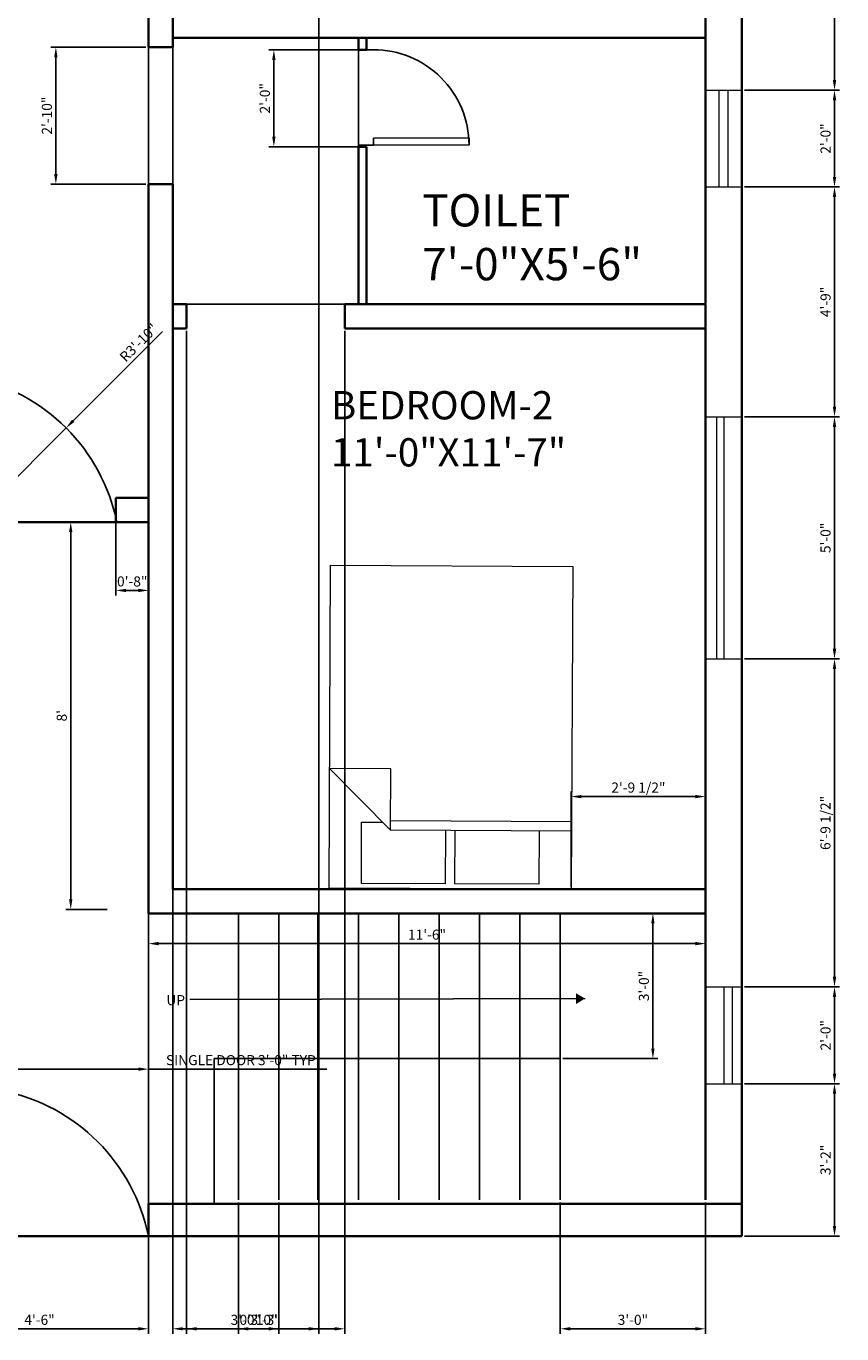
# Model space of a CAD drawing. Units: inches. Extents: x -2945 to -2182, y 3541 to 4172.
# Tile 4 of 5: x -2384 to -2182, y 3541 to 3865. Entities that reach past the tile are written whole.
import ezdxf

# ---------------------------------------------------------------- set-up
doc = ezdxf.new("R2010")
doc.units = ezdxf.units.IN
for name, color, linetype, lineweight in [('A-ANNO-DIMS', 2, 'Continuous', 18), ('A-ANNO-TEXT', 7, 'Continuous', 18), ('A-AREA-IDEN', 7, 'Continuous', 18), ('A-DOOR', 3, 'Continuous', 25), ('A-FLOR-STRS', 7, 'Continuous', 25), ('A-FURN', 9, 'Continuous', 18), ('A-GLAZ', 4, 'Continuous', 18), ('A-WALL', 7, 'Continuous', 35)]:
    doc.layers.add(name, color=color, linetype=linetype, lineweight=lineweight)
doc.styles.get("Standard").update_dxf_attribs({"font": 'arial.ttf'})
doc.dimstyles.new('ISO-25', dxfattribs={"dimtxt": 2.5, "dimasz": 2.5, "dimexe": 1.25, "dimexo": 0.625, "dimtad": 1, "dimdec": 0, "dimlunit": 3, "dimtxsty": 'Standard', "dimcen": 2.5, "dimadec": 0, "dimazin": 0, "dimtfac": 1, "dimtdec": 0, "dimtmove": 0, "dimatfit": 3, "dimfxl": 1, "dimarcsym": 0})

# ---------------------------------------------------------------- blocks, each defined once
blk = doc.blocks.new('Bed - Queen')
for p, q in [((0, -80.00003), (0, 0)), ((0, 0), (59.99999, 0)), ((59.99999, 0), (59.99999, -80.00003)), ((7.99999, -1.2), (28.79998, -1.2)), ((7.99999, -14.4), (7.99999, -1.2)), ((28.79998, -1.2), (28.79998, -14.4)), ((31.19999, -1.2), (51.99999, -1.2)), ((31.19999, -14.4), (31.19999, -1.2)), ((51.99999, -1.2), (51.99999, -16.4)), ((0, -14.4), (44.8, -14.4)), ((59.99999, -29.6), (44.8, -14.4)), ((44.8, -14.4), (44.8, -29.6)), ((44.8, -16.8), (0, -16.8)), ((51.99999, -16.4), (46.79936, -16.4)), ((44.8, -29.6), (59.99999, -29.6)), ((59.99999, -80.00003), (0, -80.00003))]:
    blk.add_line(p, q)
blk = doc.blocks.new('*U5')
for p, q in [((-600, 0), (-600, -100)), ((0, 0), (0, -100))]:
    blk.add_line(p, q)
blk.add_lwpolyline([(0, 0), (0, 600), (-43.75, 600), (-43.75, 0)], close=True)
blk.add_arc((0, 0), 600, 90, 180)
blk = doc.blocks.new('*D7')
at = {"layer": 'A-ANNO-DIMS', "color": 0, "lineweight": -2, "transparency": 16777216}
for p, q in [((-2354.05, 3636.42), (-2354.05, 3639.34)), ((-2218.55, 3638.09), (-2351.55, 3638.09)), ((-2216.05, 3636.42), (-2216.05, 3639.34))]:
    blk.add_line(p, q, dxfattribs=at)
at = {"layer": 'A-ANNO-DIMS', "color": 0, "transparency": 16777216}
for points in [[(-2351.55, 3638.51), (-2351.55, 3637.67), (-2354.05, 3638.09)], [(-2218.55, 3638.51), (-2218.55, 3637.67), (-2216.05, 3638.09)]]:
    blk.add_solid(points, dxfattribs=at)
at = {"layer": 'Defpoints', "color": 0, "transparency": 16777216}
for p in [(-2354.05, 3638.09), (-2354.05, 3635.8), (-2216.05, 3635.8)]:
    blk.add_point(p, dxfattribs=at)
at = {"layer": 'A-ANNO-DIMS', "color": 0, "transparency": 16777216, "insert": (-2285.05, 3639.99), "char_height": 2.5, "attachment_point": 5}
blk.add_mtext('11\'-6"', dxfattribs=at)
blk = doc.blocks.new('*D8')
at = {"layer": 'A-ANNO-DIMS', "color": 0, "lineweight": -2, "transparency": 16777216}
for p, q in [((-2362.73, 3742.58), (-2374.56, 3742.58)), ((-2373.31, 3740.08), (-2373.31, 3649.07)), ((-2364.29, 3646.57), (-2374.56, 3646.57))]:
    blk.add_line(p, q, dxfattribs=at)
at = {"layer": 'A-ANNO-DIMS', "color": 0, "transparency": 16777216}
for points in [[(-2373.73, 3740.08), (-2372.9, 3740.08), (-2373.31, 3742.58)], [(-2373.73, 3649.07), (-2372.9, 3649.07), (-2373.31, 3646.57)]]:
    blk.add_solid(points, dxfattribs=at)
at = {"layer": 'Defpoints', "color": 0, "transparency": 16777216}
for p in [(-2362.11, 3742.58), (-2373.31, 3646.57), (-2363.67, 3646.57)]:
    blk.add_point(p, dxfattribs=at)
at = {"layer": 'A-ANNO-DIMS', "color": 0, "transparency": 16777216, "insert": (-2375.22, 3694.57), "char_height": 2.5, "attachment_point": 5, "rotation": 90}
blk.add_mtext("8'", dxfattribs=at)
blk = doc.blocks.new('DOOR-SINGLE-36IN')
for p, q in [((0, 0), (0, 36)), ((1, 0), (1, 36))]:
    blk.add_line(p, q)
blk.add_arc((-9.18, -9.18), 46.1, 11.4852, 78.5148)
blk = doc.blocks.new('*D18')
at = {"layer": 'A-ANNO-DIMS', "color": 0, "lineweight": -2, "transparency": 16777216}
for p, q in [((-2390.05, 3602.2), (-2390.05, 3608.23)), ((-2354.05, 3602.2), (-2354.05, 3608.23)), ((-2387.55, 3606.98), (-2356.55, 3606.98)), ((-2354.05, 3606.98), (-2309.84, 3606.98))]:
    blk.add_line(p, q, dxfattribs=at)
at = {"layer": 'A-ANNO-DIMS', "color": 0, "transparency": 16777216}
for points in [[(-2387.55, 3607.39), (-2387.55, 3606.56), (-2390.05, 3606.98)], [(-2356.55, 3607.39), (-2356.55, 3606.56), (-2354.05, 3606.98)]]:
    blk.add_solid(points, dxfattribs=at)
at = {"layer": 'Defpoints', "color": 0, "transparency": 16777216}
for p in [(-2354.05, 3606.98), (-2390.05, 3601.58), (-2354.05, 3601.58)]:
    blk.add_point(p, dxfattribs=at)
at = {"layer": 'A-ANNO-DIMS', "color": 0, "transparency": 16777216, "insert": (-2330.7, 3608.89), "char_height": 2.5, "attachment_point": 5}
blk.add_mtext('SINGLE DOOR 3\'-0" TYP.', dxfattribs=at)
blk = doc.blocks.new('*D33')
at = {"layer": 'A-ANNO-DIMS', "color": 0, "lineweight": -2, "transparency": 16777216}
for p, q in [((-2206.42, 3603.38), (-2182.85, 3603.38)), ((-2184.1, 3568.08), (-2184.1, 3600.88)), ((-2206.42, 3565.58), (-2182.85, 3565.58))]:
    blk.add_line(p, q, dxfattribs=at)
at = {"layer": 'A-ANNO-DIMS', "color": 0, "transparency": 16777216}
for points in [[(-2184.52, 3600.88), (-2183.68, 3600.88), (-2184.1, 3603.38)], [(-2184.52, 3568.08), (-2183.68, 3568.08), (-2184.1, 3565.58)]]:
    blk.add_solid(points, dxfattribs=at)
at = {"layer": 'Defpoints', "color": 0, "transparency": 16777216}
for p in [(-2207.05, 3603.38), (-2184.1, 3603.38), (-2207.05, 3565.58)]:
    blk.add_point(p, dxfattribs=at)
at = {"layer": 'A-ANNO-DIMS', "color": 0, "transparency": 16777216, "insert": (-2186, 3584.48), "char_height": 2.5, "attachment_point": 5, "rotation": 90}
blk.add_mtext('3\'-2"', dxfattribs=at)
blk = doc.blocks.new('*D34')
at = {"layer": 'A-ANNO-DIMS', "color": 0, "lineweight": -2, "transparency": 16777216}
for p, q in [((-2206.42, 3627.38), (-2182.85, 3627.38)), ((-2184.1, 3605.88), (-2184.1, 3624.88)), ((-2206.42, 3603.38), (-2182.85, 3603.38))]:
    blk.add_line(p, q, dxfattribs=at)
at = {"layer": 'A-ANNO-DIMS', "color": 0, "transparency": 16777216}
for points in [[(-2184.52, 3624.88), (-2183.68, 3624.88), (-2184.1, 3627.38)], [(-2184.52, 3605.88), (-2183.68, 3605.88), (-2184.1, 3603.38)]]:
    blk.add_solid(points, dxfattribs=at)
at = {"layer": 'Defpoints', "color": 0, "transparency": 16777216}
for p in [(-2207.05, 3627.38), (-2184.1, 3627.38), (-2207.05, 3603.38)]:
    blk.add_point(p, dxfattribs=at)
at = {"layer": 'A-ANNO-DIMS', "color": 0, "transparency": 16777216, "insert": (-2186, 3615.38), "char_height": 2.5, "attachment_point": 5, "rotation": 90}
blk.add_mtext('2\'-0"', dxfattribs=at)
blk = doc.blocks.new('*D35')
at = {"layer": 'A-ANNO-DIMS', "color": 0, "lineweight": -2, "transparency": 16777216}
for p, q in [((-2206.42, 3708.65), (-2182.85, 3708.65)), ((-2184.1, 3629.88), (-2184.1, 3706.15)), ((-2206.42, 3627.38), (-2182.85, 3627.38))]:
    blk.add_line(p, q, dxfattribs=at)
at = {"layer": 'A-ANNO-DIMS', "color": 0, "transparency": 16777216}
for points in [[(-2184.52, 3706.15), (-2183.68, 3706.15), (-2184.1, 3708.65)], [(-2184.52, 3629.88), (-2183.68, 3629.88), (-2184.1, 3627.38)]]:
    blk.add_solid(points, dxfattribs=at)
at = {"layer": 'Defpoints', "color": 0, "transparency": 16777216}
for p in [(-2207.05, 3708.65), (-2184.1, 3708.65), (-2207.05, 3627.38)]:
    blk.add_point(p, dxfattribs=at)
at = {"layer": 'A-ANNO-DIMS', "color": 0, "transparency": 16777216, "insert": (-2186.02, 3668.01), "char_height": 2.5, "attachment_point": 5, "rotation": 90}
blk.add_mtext('6\'-9 1/2"', dxfattribs=at)
blk = doc.blocks.new('*D36')
at = {"layer": 'A-ANNO-DIMS', "color": 0, "lineweight": -2, "transparency": 16777216}
for p, q in [((-2206.42, 3768.65), (-2182.85, 3768.65)), ((-2184.1, 3711.15), (-2184.1, 3766.15)), ((-2206.42, 3708.65), (-2182.85, 3708.65))]:
    blk.add_line(p, q, dxfattribs=at)
at = {"layer": 'A-ANNO-DIMS', "color": 0, "transparency": 16777216}
for points in [[(-2184.52, 3766.15), (-2183.68, 3766.15), (-2184.1, 3768.65)], [(-2184.52, 3711.15), (-2183.68, 3711.15), (-2184.1, 3708.65)]]:
    blk.add_solid(points, dxfattribs=at)
at = {"layer": 'Defpoints', "color": 0, "transparency": 16777216}
for p in [(-2207.05, 3768.65), (-2184.1, 3768.65), (-2207.05, 3708.65)]:
    blk.add_point(p, dxfattribs=at)
at = {"layer": 'A-ANNO-DIMS', "color": 0, "transparency": 16777216, "insert": (-2186, 3738.65), "char_height": 2.5, "attachment_point": 5, "rotation": 90}
blk.add_mtext('5\'-0"', dxfattribs=at)
blk = doc.blocks.new('*D37')
at = {"layer": 'A-ANNO-DIMS', "color": 0, "lineweight": -2, "transparency": 16777216}
for p, q in [((-2206.42, 3825.62), (-2182.85, 3825.62)), ((-2184.1, 3771.15), (-2184.1, 3823.12)), ((-2206.42, 3768.65), (-2182.85, 3768.65))]:
    blk.add_line(p, q, dxfattribs=at)
at = {"layer": 'A-ANNO-DIMS', "color": 0, "transparency": 16777216}
for points in [[(-2184.52, 3823.12), (-2183.68, 3823.12), (-2184.1, 3825.62)], [(-2184.52, 3771.15), (-2183.68, 3771.15), (-2184.1, 3768.65)]]:
    blk.add_solid(points, dxfattribs=at)
at = {"layer": 'Defpoints', "color": 0, "transparency": 16777216}
for p in [(-2207.05, 3825.62), (-2184.1, 3825.62), (-2207.05, 3768.65)]:
    blk.add_point(p, dxfattribs=at)
at = {"layer": 'A-ANNO-DIMS', "color": 0, "transparency": 16777216, "insert": (-2186, 3797.13), "char_height": 2.5, "attachment_point": 5, "rotation": 90}
blk.add_mtext('4\'-9"', dxfattribs=at)
blk = doc.blocks.new('*D38')
at = {"layer": 'A-ANNO-DIMS', "color": 0, "lineweight": -2, "transparency": 16777216}
for p, q in [((-2206.42, 3849.62), (-2182.85, 3849.62)), ((-2184.1, 3828.12), (-2184.1, 3847.12)), ((-2206.42, 3825.62), (-2182.85, 3825.62))]:
    blk.add_line(p, q, dxfattribs=at)
at = {"layer": 'A-ANNO-DIMS', "color": 0, "transparency": 16777216}
for points in [[(-2184.52, 3847.12), (-2183.68, 3847.12), (-2184.1, 3849.62)], [(-2184.52, 3828.12), (-2183.68, 3828.12), (-2184.1, 3825.62)]]:
    blk.add_solid(points, dxfattribs=at)
at = {"layer": 'Defpoints', "color": 0, "transparency": 16777216}
for p in [(-2207.05, 3849.62), (-2184.1, 3849.62), (-2207.05, 3825.62)]:
    blk.add_point(p, dxfattribs=at)
at = {"layer": 'A-ANNO-DIMS', "color": 0, "transparency": 16777216, "insert": (-2186, 3837.62), "char_height": 2.5, "attachment_point": 5, "rotation": 90}
blk.add_mtext('2\'-0"', dxfattribs=at)
blk = doc.blocks.new('*D39')
at = {"layer": 'A-ANNO-DIMS', "color": 0, "lineweight": -2, "transparency": 16777216}
for p, q in [((-2206.42, 3918.54), (-2182.85, 3918.54)), ((-2184.1, 3852.12), (-2184.1, 3916.04)), ((-2206.42, 3849.62), (-2182.85, 3849.62))]:
    blk.add_line(p, q, dxfattribs=at)
at = {"layer": 'A-ANNO-DIMS', "color": 0, "transparency": 16777216}
for points in [[(-2184.52, 3916.04), (-2183.68, 3916.04), (-2184.1, 3918.54)], [(-2184.52, 3852.12), (-2183.68, 3852.12), (-2184.1, 3849.62)]]:
    blk.add_solid(points, dxfattribs=at)
at = {"layer": 'Defpoints', "color": 0, "transparency": 16777216}
for p in [(-2207.05, 3918.54), (-2184.1, 3918.54), (-2207.05, 3849.62)]:
    blk.add_point(p, dxfattribs=at)
at = {"layer": 'A-ANNO-DIMS', "color": 0, "transparency": 16777216, "insert": (-2186, 3884.08), "char_height": 2.5, "attachment_point": 5, "rotation": 90}
blk.add_mtext('5\'-9"', dxfattribs=at)
blk = doc.blocks.new('*D41')
at = {"layer": 'A-ANNO-DIMS', "color": 0, "lineweight": -2, "transparency": 16777216}
for p, q in [((-2408.05, 3920.95), (-2408.05, 3541.38)), ((-2354.05, 3920.95), (-2354.05, 3541.38)), ((-2405.55, 3542.63), (-2356.55, 3542.63))]:
    blk.add_line(p, q, dxfattribs=at)
at = {"layer": 'A-ANNO-DIMS', "color": 0, "transparency": 16777216}
for points in [[(-2405.55, 3543.04), (-2405.55, 3542.21), (-2408.05, 3542.63)], [(-2356.55, 3543.04), (-2356.55, 3542.21), (-2354.05, 3542.63)]]:
    blk.add_solid(points, dxfattribs=at)
at = {"layer": 'Defpoints', "color": 0, "transparency": 16777216}
for p in [(-2408.05, 3921.58), (-2354.05, 3921.58), (-2354.05, 3542.63)]:
    blk.add_point(p, dxfattribs=at)
at = {"layer": 'A-ANNO-DIMS', "color": 0, "transparency": 16777216, "insert": (-2381.05, 3544.53), "char_height": 2.5, "attachment_point": 5}
blk.add_mtext('4\'-6"', dxfattribs=at)
blk = doc.blocks.new('*D48')
at = {"layer": 'A-ANNO-DIMS', "color": 0, "lineweight": -2, "transparency": 16777216}
for p, q in [((-2300.67, 3859.61), (-2324.24, 3859.61)), ((-2323, 3838.08), (-2323, 3857.11)), ((-2300.67, 3835.57), (-2324.25, 3835.58))]:
    blk.add_line(p, q, dxfattribs=at)
at = {"layer": 'A-ANNO-DIMS', "color": 0, "transparency": 16777216}
for points in [[(-2323.41, 3857.11), (-2322.58, 3857.11), (-2322.99, 3859.61)], [(-2323.41, 3838.08), (-2322.58, 3838.08), (-2323, 3835.58)]]:
    blk.add_solid(points, dxfattribs=at)
at = {"layer": 'Defpoints', "color": 0, "transparency": 16777216}
for p in [(-2322.99, 3859.61), (-2300.04, 3859.61), (-2300.05, 3835.57)]:
    blk.add_point(p, dxfattribs=at)
at = {"layer": 'A-ANNO-DIMS', "color": 0, "transparency": 16777216, "insert": (-2324.9, 3847.6), "char_height": 2.5, "attachment_point": 5, "rotation": 89.9911}
blk.add_mtext('2\'-0"', dxfattribs=at)
blk = doc.blocks.new('*D50')
at = {"layer": 'A-ANNO-DIMS', "color": 0, "lineweight": -2, "transparency": 16777216}
for p, q in [((-2354.67, 3860.25), (-2378.25, 3860.25)), ((-2377, 3828.85), (-2377, 3857.75)), ((-2354.67, 3826.35), (-2378.25, 3826.35))]:
    blk.add_line(p, q, dxfattribs=at)
at = {"layer": 'A-ANNO-DIMS', "color": 0, "transparency": 16777216}
for points in [[(-2377.42, 3857.75), (-2376.58, 3857.75), (-2377, 3860.25)], [(-2377.42, 3828.85), (-2376.58, 3828.85), (-2377, 3826.35)]]:
    blk.add_solid(points, dxfattribs=at)
at = {"layer": 'Defpoints', "color": 0, "transparency": 16777216}
for p in [(-2377, 3860.25), (-2354.05, 3860.25), (-2354.05, 3826.35)]:
    blk.add_point(p, dxfattribs=at)
at = {"layer": 'A-ANNO-DIMS', "color": 0, "transparency": 16777216, "insert": (-2378.9, 3843.3), "char_height": 2.5, "attachment_point": 5, "rotation": 90}
blk.add_mtext('2\'-10"', dxfattribs=at)
blk = doc.blocks.new('*D51')
at = {"layer": 'A-ANNO-DIMS', "color": 0, "lineweight": -2, "transparency": 16777216}
for p, q in [((-2344.65, 3789.95), (-2344.65, 3541.38)), ((-2305.42, 3789.95), (-2305.42, 3541.38)), ((-2342.15, 3542.63), (-2307.92, 3542.63))]:
    blk.add_line(p, q, dxfattribs=at)
at = {"layer": 'A-ANNO-DIMS', "color": 0, "transparency": 16777216}
for points in [[(-2342.15, 3543.04), (-2342.15, 3542.21), (-2344.65, 3542.63)], [(-2307.92, 3543.04), (-2307.92, 3542.21), (-2305.42, 3542.63)]]:
    blk.add_solid(points, dxfattribs=at)
at = {"layer": 'Defpoints', "color": 0, "transparency": 16777216}
for p in [(-2344.65, 3790.58), (-2305.42, 3790.58), (-2305.42, 3542.63)]:
    blk.add_point(p, dxfattribs=at)
at = {"layer": 'A-ANNO-DIMS', "color": 0, "transparency": 16777216, "insert": (-2325.04, 3544.53), "char_height": 2.5, "attachment_point": 5}
blk.add_mtext('3\'-3"', dxfattribs=at)
blk = doc.blocks.new('*D52')
at = {"layer": 'A-ANNO-DIMS', "color": 0, "lineweight": -2, "transparency": 16777216}
for p, q in [((-2252.05, 3573.95), (-2252.05, 3541.38)), ((-2216.05, 3573.95), (-2216.05, 3541.38)), ((-2249.55, 3542.63), (-2218.55, 3542.63))]:
    blk.add_line(p, q, dxfattribs=at)
at = {"layer": 'A-ANNO-DIMS', "color": 0, "transparency": 16777216}
for points in [[(-2249.55, 3543.04), (-2249.55, 3542.21), (-2252.05, 3542.63)], [(-2218.55, 3543.04), (-2218.55, 3542.21), (-2216.05, 3542.63)]]:
    blk.add_solid(points, dxfattribs=at)
at = {"layer": 'Defpoints', "color": 0, "transparency": 16777216}
for p in [(-2252.05, 3574.58), (-2216.05, 3574.58), (-2216.05, 3542.63)]:
    blk.add_point(p, dxfattribs=at)
at = {"layer": 'A-ANNO-DIMS', "color": 0, "transparency": 16777216, "insert": (-2234.05, 3544.53), "char_height": 2.5, "attachment_point": 5}
blk.add_mtext('3\'-0"', dxfattribs=at)
blk = doc.blocks.new('*D53')
at = {"layer": 'A-ANNO-DIMS', "color": 0, "lineweight": -2, "transparency": 16777216}
for p, q in [((-2331.79, 3573.95), (-2331.79, 3541.38)), ((-2321.79, 3573.95), (-2321.79, 3541.38)), ((-2329.29, 3542.63), (-2324.29, 3542.63))]:
    blk.add_line(p, q, dxfattribs=at)
at = {"layer": 'A-ANNO-DIMS', "color": 0, "transparency": 16777216}
for points in [[(-2329.29, 3543.04), (-2329.29, 3542.21), (-2331.79, 3542.63)], [(-2324.29, 3543.04), (-2324.29, 3542.21), (-2321.79, 3542.63)]]:
    blk.add_solid(points, dxfattribs=at)
at = {"layer": 'Defpoints', "color": 0, "transparency": 16777216}
for p in [(-2331.79, 3574.58), (-2321.79, 3574.58), (-2321.79, 3542.63)]:
    blk.add_point(p, dxfattribs=at)
at = {"layer": 'A-ANNO-DIMS', "color": 0, "transparency": 16777216, "insert": (-2326.79, 3544.53), "char_height": 2.5, "attachment_point": 5}
blk.add_mtext('0\'-10"', dxfattribs=at)
blk = doc.blocks.new('*D54')
at = {"layer": 'A-ANNO-DIMS', "color": 0, "lineweight": -2, "transparency": 16777216}
for p, q in [((-2251.42, 3645.58), (-2227.85, 3645.58)), ((-2229.1, 3643.08), (-2229.1, 3612.08)), ((-2251.42, 3609.58), (-2227.85, 3609.58))]:
    blk.add_line(p, q, dxfattribs=at)
at = {"layer": 'A-ANNO-DIMS', "color": 0, "transparency": 16777216}
for points in [[(-2229.52, 3643.08), (-2228.68, 3643.08), (-2229.1, 3645.58)], [(-2229.52, 3612.08), (-2228.68, 3612.08), (-2229.1, 3609.58)]]:
    blk.add_solid(points, dxfattribs=at)
at = {"layer": 'Defpoints', "color": 0, "transparency": 16777216}
for p in [(-2252.05, 3645.58), (-2252.05, 3609.58), (-2229.1, 3609.58)]:
    blk.add_point(p, dxfattribs=at)
at = {"layer": 'A-ANNO-DIMS', "color": 0, "transparency": 16777216, "insert": (-2231, 3627.58), "char_height": 2.5, "attachment_point": 5, "rotation": 90}
blk.add_mtext('3\'-0"', dxfattribs=at)
blk = doc.blocks.new('*D55')
at = {"layer": 'A-ANNO-DIMS', "color": 0, "lineweight": -2, "transparency": 16777216}
for p, q in [((-2348.05, 3999.95), (-2348.05, 3541.38)), ((-2311.84, 3998.65), (-2311.84, 3541.38)), ((-2345.55, 3542.63), (-2314.34, 3542.63))]:
    blk.add_line(p, q, dxfattribs=at)
at = {"layer": 'A-ANNO-DIMS', "color": 0, "transparency": 16777216}
for points in [[(-2345.55, 3543.04), (-2345.55, 3542.21), (-2348.05, 3542.63)], [(-2314.34, 3543.04), (-2314.34, 3542.21), (-2311.84, 3542.63)]]:
    blk.add_solid(points, dxfattribs=at)
at = {"layer": 'Defpoints', "color": 0, "transparency": 16777216}
for p in [(-2348.05, 4000.58), (-2311.84, 3999.28), (-2311.84, 3542.63)]:
    blk.add_point(p, dxfattribs=at)
at = {"layer": 'A-ANNO-DIMS', "color": 0, "transparency": 16777216, "insert": (-2329.94, 3544.53), "char_height": 2.5, "attachment_point": 5}
blk.add_mtext('3\'-0"', dxfattribs=at)
blk = doc.blocks.new('*D56')
at = {"layer": 'A-ANNO-DIMS', "color": 0, "lineweight": -2, "transparency": 16777216}
for p, q in [((-2249.33, 3652.2), (-2249.33, 3675.78)), ((-2216.05, 3652.2), (-2216.05, 3675.78)), ((-2246.83, 3674.53), (-2218.55, 3674.53))]:
    blk.add_line(p, q, dxfattribs=at)
at = {"layer": 'A-ANNO-DIMS', "color": 0, "transparency": 16777216}
for points in [[(-2246.83, 3674.94), (-2246.83, 3674.11), (-2249.33, 3674.53)], [(-2218.55, 3674.94), (-2218.55, 3674.11), (-2216.05, 3674.53)]]:
    blk.add_solid(points, dxfattribs=at)
at = {"layer": 'Defpoints', "color": 0, "transparency": 16777216}
for p in [(-2216.05, 3674.53), (-2249.33, 3651.58), (-2216.05, 3651.58)]:
    blk.add_point(p, dxfattribs=at)
at = {"layer": 'A-ANNO-DIMS', "color": 0, "transparency": 16777216, "insert": (-2232.69, 3676.44), "char_height": 2.5, "attachment_point": 5}
blk.add_mtext('2\'-9 1/2"', dxfattribs=at)
blk = doc.blocks.new('*D57')
at = {"layer": 'A-ANNO-DIMS', "color": 0, "lineweight": -2, "transparency": 16777216}
for p, q in [((-2362.11, 3747.95), (-2362.11, 3724.38)), ((-2354.05, 3747.95), (-2354.05, 3724.38)), ((-2356.55, 3725.63), (-2359.61, 3725.63))]:
    blk.add_line(p, q, dxfattribs=at)
at = {"layer": 'A-ANNO-DIMS', "color": 0, "transparency": 16777216}
for points in [[(-2359.61, 3726.04), (-2359.61, 3725.21), (-2362.11, 3725.63)], [(-2356.55, 3726.04), (-2356.55, 3725.21), (-2354.05, 3725.63)]]:
    blk.add_solid(points, dxfattribs=at)
at = {"layer": 'Defpoints', "color": 0, "transparency": 16777216}
for p in [(-2362.11, 3748.58), (-2354.05, 3748.58), (-2362.11, 3725.63)]:
    blk.add_point(p, dxfattribs=at)
at = {"layer": 'A-ANNO-DIMS', "color": 0, "transparency": 16777216, "insert": (-2358.08, 3727.53), "char_height": 2.5, "attachment_point": 5}
blk.add_mtext('0\'-8"', dxfattribs=at)
blk = doc.blocks.new('*D77')
at = {"layer": 'A-ANNO-DIMS', "color": 0, "lineweight": -2, "transparency": 16777216}
for p, q in [((-2350.58, 3789.78), (-2372.69, 3767.66)), ((-2407.06, 3733.29), (-2374.46, 3765.89))]:
    blk.add_line(p, q, dxfattribs=at)
at = {"layer": 'A-ANNO-DIMS', "color": 0, "transparency": 16777216}
blk.add_solid([(-2372.99, 3767.96), (-2372.4, 3767.37), (-2374.46, 3765.89)], dxfattribs=at)
at = {"layer": 'Defpoints', "color": 0, "transparency": 16777216}
for p in [(-2374.46, 3765.89), (-2407.06, 3733.29)]:
    blk.add_point(p, dxfattribs=at)
at = {"layer": 'A-ANNO-DIMS', "color": 0, "transparency": 16777216, "insert": (-2356.24, 3786.8), "char_height": 2.5, "attachment_point": 5, "rotation": 44.9998}
blk.add_mtext('R3\'-10"', dxfattribs=at)

msp = doc.modelspace()

# ---------------------------------------------------------------- linework, layer by layer
at = {"layer": 'A-DOOR'}
for p, q in [((-2302.02, 3835.57), (-2302.02, 3859.57)), ((-2344.65, 3796.58), (-2305.42, 3796.58))]:
    msp.add_line(p, q, dxfattribs=at)
at = {"layer": 'A-FLOR-STRS'}
for p, q in [((-2331.79, 3645.58), (-2331.79, 3574.58)), ((-2321.79, 3645.58), (-2321.79, 3574.58)), ((-2312.11, 3645.58), (-2312.11, 3574.58)), ((-2302.02, 3645.58), (-2302.02, 3574.58)), ((-2292.05, 3645.58), (-2292.05, 3574.58)), ((-2282.05, 3645.58), (-2282.05, 3574.58)), ((-2272.05, 3645.58), (-2272.05, 3574.58)), ((-2272.05, 3645.58), (-2272.05, 3574.58)), ((-2262.05, 3645.58), (-2262.05, 3574.58)), ((-2262.05, 3645.58), (-2262.05, 3574.58)), ((-2252.05, 3645.58), (-2252.05, 3574.58)), ((-2343.79, 3624.21), (-2245.91, 3624.47)), ((-2331.79, 3609.58), (-2337.77, 3609.58)), ((-2337.77, 3609.58), (-2337.77, 3573.58)), ((-2252.05, 3609.58), (-2331.79, 3609.58))]:
    msp.add_line(p, q, dxfattribs=at)
msp.add_lwpolyline([(-2245.91, 3624.47, 0, 2.68, 0), (-2248.15, 3624.46, 2.68, 2.68, 0)], format="xyseb", dxfattribs=at)
at = {"layer": 'A-GLAZ'}
for p, q in [((-2216.05, 3849.62), (-2207.05, 3849.62)), ((-2212.73, 3849.62), (-2212.73, 3825.62)), ((-2210.56, 3849.62), (-2210.56, 3825.62)), ((-2216.05, 3825.62), (-2207.05, 3825.62)), ((-2216.05, 3768.65), (-2207.05, 3768.65)), ((-2213.37, 3768.65), (-2213.37, 3708.65)), ((-2211.55, 3768.65), (-2211.55, 3708.65)), ((-2216.05, 3708.65), (-2207.05, 3708.65)), ((-2216.05, 3627.38), (-2207.05, 3627.38)), ((-2211.55, 3627.38), (-2211.55, 3603.38)), ((-2209.48, 3627.38), (-2209.48, 3603.38)), ((-2216.05, 3603.38), (-2207.05, 3603.38))]:
    msp.add_line(p, q, dxfattribs=at)
at = {"layer": 'A-WALL'}
for p, q in [((-2207.05, 4009.58), (-2207.05, 3565.58)), ((-2216.05, 4000.58), (-2216.05, 3574.58)), ((-2354.05, 3860.25), (-2354.05, 3872.23)), ((-2348.05, 3860.25), (-2348.05, 3872.23)), ((-2354.05, 3860.25), (-2348.05, 3860.25)), ((-2348.05, 3862.58), (-2216.05, 3862.58)), ((-2302.02, 3862.58), (-2302.02, 3859.57)), ((-2300.05, 3862.58), (-2300.05, 3859.57)), ((-2302.02, 3859.57), (-2300.05, 3859.57)), ((-2302.02, 3835.57), (-2300.05, 3835.57)), ((-2302.02, 3835.57), (-2302.02, 3796.58)), ((-2300.05, 3835.57), (-2300.05, 3796.58)), ((-2354.05, 3645.58), (-2354.05, 3826.35)), ((-2354.05, 3826.35), (-2348.05, 3826.35)), ((-2348.05, 3651.58), (-2348.05, 3826.35)), ((-2348.05, 3796.58), (-2344.65, 3796.58)), ((-2344.65, 3796.58), (-2344.65, 3790.58)), ((-2305.42, 3796.58), (-2305.42, 3790.58)), ((-2305.42, 3796.58), (-2216.05, 3796.58)), ((-2348.05, 3790.58), (-2344.65, 3790.58)), ((-2305.42, 3790.58), (-2216.05, 3790.58)), ((-2362.11, 3748.58), (-2362.11, 3742.58)), ((-2362.11, 3748.58), (-2354.05, 3748.58)), ((-2522.05, 3742.58), (-2354.05, 3742.58)), ((-2348.05, 3651.58), (-2216.05, 3651.58)), ((-2354.05, 3645.58), (-2216.05, 3645.58)), ((-2207.05, 3573.58), (-2354.05, 3573.58)), ((-2354.05, 3573.58), (-2354.05, 3565.58)), ((-2207.05, 3565.58), (-2531.05, 3565.58))]:
    msp.add_line(p, q, dxfattribs=at)

# ---------------------------------------------------------------- block references
at = {"layer": 'A-DOOR', "xscale": 0.0393700787401575, "yscale": 0.0393700787401575, "zscale": 0.0393700787401575, "rotation": 270.1211645851394}
msp.add_blockref('*U5', (-2298.27, 3835.99), dxfattribs=at)
at = {"layer": 'A-DOOR'}
for p in [(-2397.88, 3742.47), (-2390.05, 3565.57)]:
    msp.add_blockref('DOOR-SINGLE-36IN', p, dxfattribs=at)
at = {"layer": 'A-FURN', "rotation": 179.7397650528711}
msp.add_blockref('Bed - Queen', (-2249.33, 3651.58), dxfattribs=at)

# ---------------------------------------------------------------- texts
at = {"layer": 'A-ANNO-TEXT', "insert": (-2349.62, 3625.33), "char_height": 2.5, "attachment_point": 1}
msp.add_mtext_dynamic_manual_height_columns('UP', width=10.3268, gutter_width=12.5, heights=[0], dxfattribs=at)
at = {"layer": 'A-AREA-IDEN', "attachment_point": 1}
for s, width, heights, insert, char_height in [('TOILET\\P7\'-0"X5\'-6"', 51.4369, [29.22], (-2286.25, 3823.83), 8), ('BEDROOM-2\\P11\'-0"X11\'-7"', 36.5253, [0], (-2308.85, 3775.02), 7)]:
    msp.add_mtext_dynamic_manual_height_columns(s, width=width, gutter_width=12.5, heights=heights, dxfattribs=dict(at, insert=insert, char_height=char_height))

# ---------------------------------------------------------------- dimensions: what is measured, and where the dimension line sits
at = {"layer": 'A-ANNO-DIMS'}
for base, p1, p2, override, picture, middle in [((-2311.84, 3542.63), (-2348.05, 4000.58), (-2311.84, 3999.28), {"dimdec": 1, "dimlfac": 1, "dimrnd": 0, "dimzin": 1, "dimdsep": 46, "dimlunit": 4, "dimfrac": 2}, '*D55', (-2329.94, 3544.53)), ((-2354.05, 3542.63), (-2408.05, 3921.58), (-2354.05, 3921.58), {"dimdec": 1, "dimlfac": 1, "dimrnd": 0, "dimzin": 1, "dimdsep": 46, "dimlunit": 4, "dimfrac": 2}, '*D41', (-2381.05, 3544.53)), ((-2305.42, 3542.63), (-2344.65, 3790.58), (-2305.42, 3790.58), {"dimdec": 1, "dimlfac": 1, "dimrnd": 0, "dimzin": 1, "dimdsep": 46, "dimlunit": 4, "dimfrac": 2}, '*D51', (-2325.04, 3544.53)), ((-2216.05, 3674.53), (-2249.33, 3651.58), (-2216.05, 3651.58), {"dimdec": 1, "dimlfac": 1, "dimrnd": 0, "dimzin": 1, "dimdsep": 46, "dimlunit": 4, "dimfrac": 2}, '*D56', (-2232.69, 3676.44)), ((-2354.05, 3638.09), (-2216.05, 3635.8), (-2354.05, 3635.8), {"dimclrd": 0, "dimclre": 0, "dimclrt": 0}, '*D7', (-2285.05, 3639.99)), ((-2321.79, 3542.63), (-2331.79, 3574.58), (-2321.79, 3574.58), {"dimdec": 1, "dimlfac": 1, "dimrnd": 0, "dimzin": 1, "dimdsep": 46, "dimlunit": 4, "dimfrac": 2}, '*D53', (-2326.79, 3544.53)), ((-2216.05, 3542.63), (-2252.05, 3574.58), (-2216.05, 3574.58), {"dimdec": 1, "dimlfac": 1, "dimrnd": 0, "dimzin": 1, "dimdsep": 46, "dimlunit": 4, "dimfrac": 2}, '*D52', (-2234.05, 3544.53))]:
    dim = msp.add_linear_dim(base=base, p1=p1, p2=p2, dimstyle='ISO-25', override=override, dxfattribs=at)
    dim.commit()
    dim.dimension.update_dxf_attribs({"geometry": picture, "text_midpoint": middle})
for base, p1, p2, angle, override, picture, middle in [((-2184.1, 3918.54), (-2207.05, 3849.62), (-2207.05, 3918.54), 90, {"dimdec": 1, "dimlfac": 1, "dimrnd": 0, "dimzin": 1, "dimdsep": 46, "dimlunit": 4, "dimfrac": 2}, '*D39', (-2186, 3884.08)), ((-2377, 3860.25), (-2354.05, 3826.35), (-2354.05, 3860.25), 90, {"dimdec": 1, "dimlfac": 1, "dimrnd": 0, "dimzin": 1, "dimdsep": 46, "dimlunit": 4, "dimfrac": 2}, '*D50', (-2378.9, 3843.3)), ((-2322.99, 3859.61), (-2300.05, 3835.57), (-2300.04, 3859.61), 89.9911, {"dimdec": 1, "dimlfac": 1, "dimrnd": 0, "dimzin": 1, "dimdsep": 46, "dimlunit": 4, "dimfrac": 2}, '*D48', (-2324.9, 3847.6)), ((-2184.1, 3849.62), (-2207.05, 3825.62), (-2207.05, 3849.62), 90, {"dimdec": 1, "dimlfac": 1, "dimrnd": 0, "dimzin": 1, "dimdsep": 46, "dimlunit": 4, "dimfrac": 2}, '*D38', (-2186, 3837.62)), ((-2184.1, 3825.62), (-2207.05, 3768.65), (-2207.05, 3825.62), 90, {"dimdec": 1, "dimlfac": 1, "dimrnd": 0, "dimzin": 1, "dimdsep": 46, "dimlunit": 4, "dimfrac": 2}, '*D37', (-2186, 3797.13)), ((-2184.1, 3768.65), (-2207.05, 3708.65), (-2207.05, 3768.65), 90, {"dimdec": 1, "dimlfac": 1, "dimrnd": 0, "dimzin": 1, "dimdsep": 46, "dimlunit": 4, "dimfrac": 2}, '*D36', (-2186, 3738.65)), ((-2362.11, 3725.63), (-2354.05, 3748.58), (-2362.11, 3748.58), 180, {"dimdec": 1, "dimlfac": 1, "dimrnd": 0, "dimzin": 1, "dimdsep": 46, "dimlunit": 4, "dimfrac": 2}, '*D57', (-2358.08, 3727.53)), ((-2373.31, 3646.57), (-2362.11, 3742.58), (-2363.67, 3646.57), 90, {"dimclrd": 0, "dimclre": 0, "dimclrt": 0}, '*D8', (-2375.22, 3694.57)), ((-2184.1, 3708.65), (-2207.05, 3627.38), (-2207.05, 3708.65), 90, {"dimdec": 1, "dimlfac": 1, "dimrnd": 0, "dimzin": 1, "dimdsep": 46, "dimlunit": 4, "dimfrac": 2}, '*D35', (-2186.02, 3668.01)), ((-2229.1, 3609.58), (-2252.05, 3645.58), (-2252.05, 3609.58), 270, {"dimdec": 1, "dimlfac": 1, "dimrnd": 0, "dimzin": 1, "dimdsep": 46, "dimlunit": 4, "dimfrac": 2}, '*D54', (-2231, 3627.58)), ((-2184.1, 3627.38), (-2207.05, 3603.38), (-2207.05, 3627.38), 90, {"dimdec": 1, "dimlfac": 1, "dimrnd": 0, "dimzin": 1, "dimdsep": 46, "dimlunit": 4, "dimfrac": 2}, '*D34', (-2186, 3615.38)), ((-2184.1, 3603.38), (-2207.05, 3565.58), (-2207.05, 3603.38), 90, {"dimdec": 1, "dimlfac": 1, "dimrnd": 0, "dimzin": 1, "dimdsep": 46, "dimlunit": 4, "dimfrac": 2}, '*D33', (-2186, 3584.48))]:
    dim = msp.add_linear_dim(base=base, p1=p1, p2=p2, angle=angle, dimstyle='ISO-25', override=override, dxfattribs=at)
    dim.commit()
    dim.dimension.update_dxf_attribs({"geometry": picture, "text_midpoint": middle})
dim = msp.add_radius_dim(center=(-2407.06, 3733.29), mpoint=(-2374.46, 3765.89), dimstyle='ISO-25', override={"dimdec": 1, "dimlfac": 1, "dimrnd": 0, "dimzin": 1, "dimdsep": 46, "dimlunit": 4, "dimfrac": 2}, dxfattribs=at)
dim.commit()
dim.dimension.update_dxf_attribs({"geometry": '*D77', "text_midpoint": (-2354.9, 3785.45), "dimtype": 164})
dim = msp.add_linear_dim(base=(-2354.05, 3606.98), p1=(-2390.05, 3601.58), p2=(-2354.05, 3601.58), text='SINGLE DOOR <> TYP.', dimstyle='ISO-25', override={"dimdec": 1, "dimlfac": 1, "dimrnd": 0, "dimzin": 1, "dimdsep": 46, "dimlunit": 4, "dimfrac": 2}, dxfattribs=at)
dim.commit()
dim.dimension.update_dxf_attribs({"geometry": '*D18', "text_midpoint": (-2330.7, 3608.89)})

doc.saveas('drawing.dxf')
